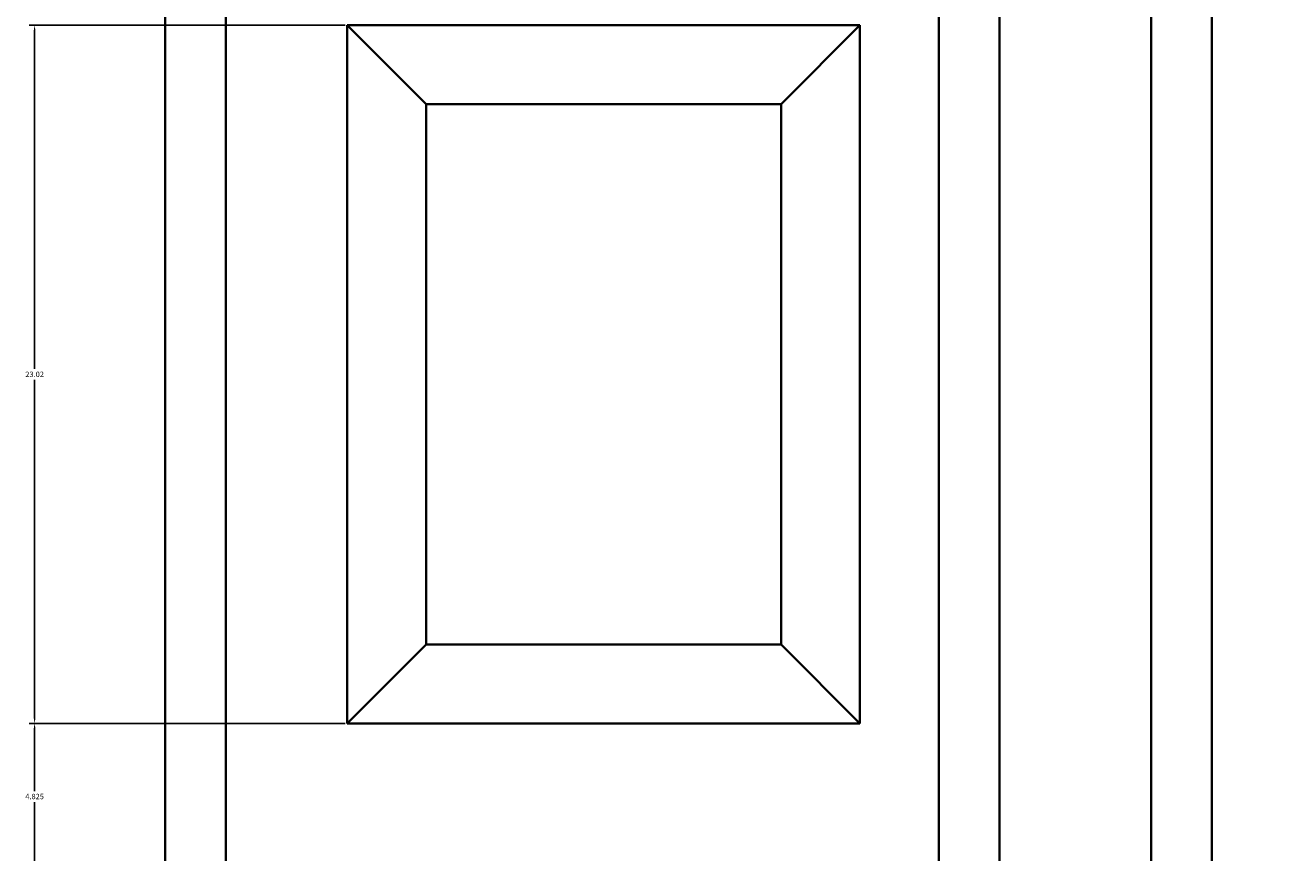
# Model space of a CAD drawing. Units: inches. Extents: x 3137 to 3299, y 1994 to 2089.
# Tile 10 of 14: x 3230 to 3272, y 2024 to 2052. Entities that reach past the tile are written whole.
import ezdxf

# ---------------------------------------------------------------- set-up
doc = ezdxf.new("R2010")
doc.units = ezdxf.units.IN
doc.header["$MEASUREMENT"] = 0
doc.layers.add('A-ANNO-DIMS', color=2, linetype='Continuous', lineweight=18)
doc.layers.add('A-DOOR', color=4, linetype='Continuous', lineweight=35)
doc.styles.get("Standard").update_dxf_attribs({"font": 'arial.ttf'})
doc.dimstyles.get("Standard").update_dxf_attribs({"dimtxt": 0.18, "dimasz": 0.18, "dimexe": 0.18, "dimexo": 0.0625, "dimgap": 0.09, "dimtad": 0, "dimtih": 1, "dimtoh": 1, "dimdec": 4, "dimzin": 0, "dimdsep": 46, "dimtxsty": 'Standard', "dimcen": 0.09, "dimadec": 0, "dimazin": 0, "dimtfac": 1, "dimtdec": 4, "dimtofl": 0, "dimtmove": 0, "dimatfit": 3, "dimfxl": 1, "dimtolj": 1, "dimtzin": 0, "dimarcsym": 0})

# ---------------------------------------------------------------- blocks, each defined once
blk = doc.blocks.new('*D68')
at = {"layer": 'A-ANNO-DIMS', "color": 0, "lineweight": -2, "transparency": 16777216}
for p, q in [((3240.441, 2028.676), (3230.019, 2028.676)), ((3230.199, 2028.496), (3230.199, 2026.445)), ((3230.199, 2024.031), (3230.199, 2026.082)), ((3240.441, 2023.851), (3230.019, 2023.851))]:
    blk.add_line(p, q, dxfattribs=at)
at = {"layer": 'A-ANNO-DIMS', "color": 0, "transparency": 16777216}
for points in [[(3230.169, 2028.496), (3230.229, 2028.496), (3230.199, 2028.676)], [(3230.169, 2024.031), (3230.229, 2024.031), (3230.199, 2023.851)]]:
    blk.add_solid(points, dxfattribs=at)
at = {"layer": 'Defpoints', "color": 0, "transparency": 16777216}
for p in [(3230.199, 2028.676), (3240.504, 2028.676), (3240.504, 2023.851)]:
    blk.add_point(p, dxfattribs=at)
at = {"layer": 'A-ANNO-DIMS', "color": 0, "transparency": 16777216, "insert": (3230.199, 2026.264), "char_height": 0.18, "attachment_point": 5}
blk.add_mtext('\\A1;4.825', dxfattribs=at)
blk = doc.blocks.new('*D69')
at = {"layer": 'A-ANNO-DIMS', "color": 0, "lineweight": -2, "transparency": 16777216}
for p, q in [((3240.441, 2051.694), (3230.019, 2051.694)), ((3230.199, 2051.514), (3230.199, 2040.367)), ((3230.199, 2028.856), (3230.199, 2040.003)), ((3240.441, 2028.676), (3230.019, 2028.676))]:
    blk.add_line(p, q, dxfattribs=at)
at = {"layer": 'A-ANNO-DIMS', "color": 0, "transparency": 16777216}
for points in [[(3230.169, 2051.514), (3230.229, 2051.514), (3230.199, 2051.694)], [(3230.169, 2028.856), (3230.229, 2028.856), (3230.199, 2028.676)]]:
    blk.add_solid(points, dxfattribs=at)
at = {"layer": 'Defpoints', "color": 0, "transparency": 16777216}
for p in [(3230.199, 2051.694), (3240.504, 2051.694), (3240.504, 2028.676)]:
    blk.add_point(p, dxfattribs=at)
at = {"layer": 'A-ANNO-DIMS', "color": 0, "transparency": 16777216, "insert": (3230.199, 2040.185), "char_height": 0.18, "attachment_point": 5}
blk.add_mtext('\\A1;23.02', dxfattribs=at)

msp = doc.modelspace()

# ---------------------------------------------------------------- linework, layer by layer
at = {"layer": 'A-DOOR'}
for p, q in [((3260.0039, 2028.6759), (3260.0039, 2082.1756)), ((3262.0039, 2028.6759), (3262.0039, 2082.1756)), ((3267.0039, 2028.6759), (3267.0039, 2082.1756)), ((3269.0039, 2028.6759), (3269.0039, 2082.1756)), ((3240.5039, 2051.6936), (3257.4039, 2051.6936)), ((3243.1039, 2049.0936), (3240.5039, 2051.6936)), ((3254.8039, 2049.0936), (3257.4039, 2051.6936)), ((3257.4039, 2028.6759), (3257.4039, 2051.6936)), ((3243.1039, 2049.0936), (3254.8039, 2049.0936)), ((3254.8039, 2031.2759), (3254.8039, 2049.0936)), ((3243.1039, 2031.2759), (3240.5039, 2028.6759)), ((3243.1039, 2031.2759), (3254.8039, 2031.2759)), ((3254.8039, 2031.2759), (3257.4039, 2028.6759)), ((3240.5039, 2028.6759), (3257.4039, 2028.6759)), ((3260.0039, 2002.1756), (3260.0039, 2028.6759)), ((3262.0039, 2002.1756), (3262.0039, 2028.6759)), ((3267.0039, 2002.1756), (3267.0039, 2028.6759)), ((3269.0039, 2002.1756), (3269.0039, 2028.6759))]:
    msp.add_line(p, q, dxfattribs=at)
for points in [[(3234.5039, 2084.1756), (3294.5039, 2084.1756), (3294.5039, 2000.1756), (3234.5039, 2000.1756)], [(3236.5039, 2082.1756), (3292.5039, 2082.1756), (3292.5039, 2002.1756), (3236.5039, 2002.1756)]]:
    msp.add_lwpolyline(points, close=True, dxfattribs=at)
for points in [[(3240.5039, 2028.6759), (3240.5039, 2051.6936)], [(3243.1039, 2031.2759), (3243.1039, 2049.0936)]]:
    msp.add_lwpolyline(points, dxfattribs=at)

# ---------------------------------------------------------------- dimensions: what is measured, and where the dimension line sits
at = {"layer": 'A-ANNO-DIMS'}
for base, p1, p2, override, picture, middle in [((3230.1989, 2051.6936), (3240.5039, 2028.6759), (3240.5039, 2051.6936), {"dimdec": 2, "dimlfac": 1, "dimrnd": 0, "dimzin": 0, "dimdsep": 46, "dimlunit": 2}, '*D69', (3230.1989, 2040.1847)), ((3230.1989, 2028.6759), (3240.5039, 2023.8512), (3240.5039, 2028.6759), {"dimdec": 3, "dimlfac": 1, "dimrnd": 0, "dimzin": 0, "dimdsep": 46, "dimlunit": 2}, '*D68', (3230.1989, 2026.2636))]:
    dim = msp.add_linear_dim(base=base, p1=p1, p2=p2, angle=90, dimstyle='Standard', override=override, dxfattribs=at)
    dim.commit()
    dim.dimension.update_dxf_attribs({"geometry": picture, "text_midpoint": middle})

doc.saveas('drawing.dxf')
